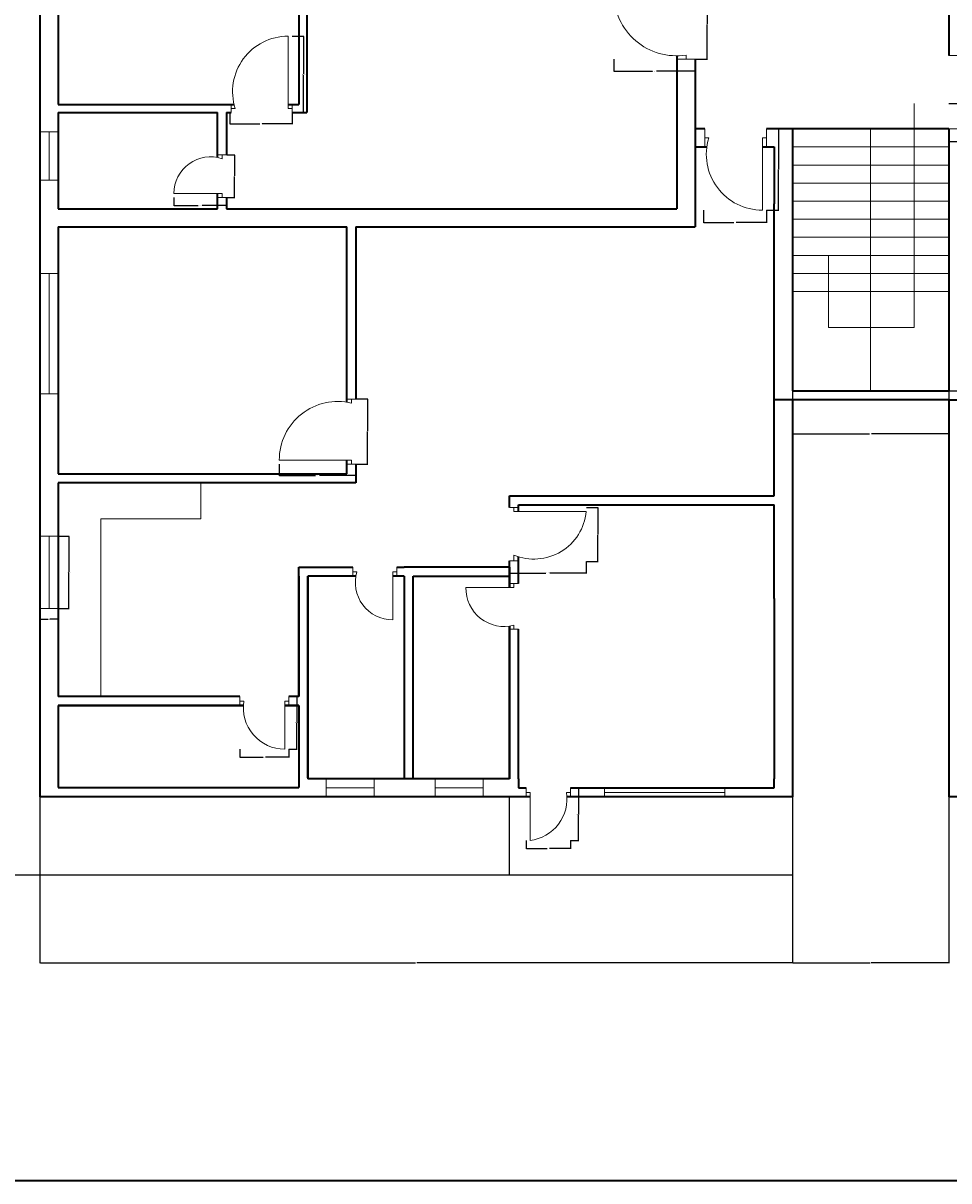
# Model space of a CAD drawing. Units: inches. Extents: x 2120 to 4013, y 1390 to 3019.
# Tile 50 of 59: x 3063 to 3525, y 1390 to 1967. Entities that reach past the tile are written whole.
import ezdxf

# ---------------------------------------------------------------- set-up
doc = ezdxf.new("R2010")
doc.units = ezdxf.units.IN
for name, color, linetype, lineweight in [('A-ANNO-DIMS', 2, 'Continuous', 18), ('A-ANNO-TTLB', 7, 'Continuous', 35), ('A-DOOR', 3, 'Continuous', 18), ('A-FLOR-CASE', 8, 'Continuous', 18), ('A-FLOR-DECK', 7, 'Continuous', 25), ('A-FLOR-STRS', 7, 'Continuous', 18), ('A-FURN', 8, 'Continuous', 13), ('A-GLAZ', 4, 'Continuous', 18), ('A-WALL', 7, 'Continuous', 35)]:
    doc.layers.add(name, color=color, linetype=linetype, lineweight=lineweight)
doc.styles.get("Standard").update_dxf_attribs({"font": 'arial.ttf'})
doc.dimstyles.get("Standard").update_dxf_attribs({"dimtxt": 0.18, "dimasz": 0.18, "dimexe": 0.18, "dimexo": 0.0625, "dimgap": 0.09, "dimtad": 0, "dimtih": 1, "dimtoh": 1, "dimdec": 4, "dimzin": 0, "dimdsep": 46, "dimtxsty": 'Standard', "dimcen": 0.09, "dimadec": 0, "dimazin": 0, "dimtfac": 1, "dimtdec": 4, "dimtofl": 0, "dimtmove": 0, "dimatfit": 3, "dimfxl": 1, "dimtolj": 1, "dimtzin": 0, "dimarcsym": 0})

# ---------------------------------------------------------------- blocks, each defined once
blk = doc.blocks.new('DOOR-SWING-24IN-108p49DEG')
for p, q in [((21.75, 21.28), (26.25, 21.28)), ((26.25, 21.28), (24, 21.28)), ((24, 21.28), (24, 19.28)), ((24, 2), (0, 2)), ((24, 0), (24, 2)), ((26.25, 0), (21.75, 0)), ((21.75, 0), (24, 0))]:
    blk.add_line(p, q)
blk.add_arc((18.22, 2), 18.22, 71.50887, 180)
blk = doc.blocks.new('DOOR-SWING-24IN-91p57DEG')
for p, q in [((0, 26.25), (0, 21.75)), ((0, 21.75), (0, 24)), ((0, 24), (2, 24)), ((2, 24), (2, 0)), ((22.12, 24), (20.12, 24)), ((22.12, 21.75), (22.12, 26.25)), ((22.12, 26.25), (22.12, 24))]:
    blk.add_line(p, q)
blk.add_arc((-0.62, 20.81), 20.98, 277.16426, 8.73852)
blk = doc.blocks.new('DOOR-SWING-24IN-105p55DEG')
for p, q in [((24, 20.82), (0, 20.82)), ((21.75, 22.82), (26.25, 22.82)), ((26.25, 22.82), (24, 22.82)), ((24, 22.82), (24, 20.82)), ((21.75, 0), (26.25, 0)), ((24, 0), (24, 2)), ((26.25, 0), (24, 0))]:
    blk.add_line(p, q)
blk.add_arc((19.15, 20.53), 19.15, 179.12074, 284.67391)
blk = doc.blocks.new('DOOR-SWING-24IN-106p83DEG')
for p, q in [((0, 21.75), (0, 26.25)), ((0, 26.25), (0, 24)), ((0, 24), (2, 24)), ((21.81, 24), (19.81, 24)), ((19.81, 24), (19.81, 0)), ((21.81, 21.75), (21.81, 26.25)), ((21.81, 26.25), (21.81, 24))]:
    blk.add_line(p, q)
blk.add_arc((19.81, 18.61), 18.61, 163.16612, 270)
blk = doc.blocks.new('DOOR-SWING-24IN-99p42DEG')
for p, q in [((0, 26.25), (0, 21.75)), ((0, 21.75), (0, 24)), ((0, 24), (2, 24)), ((24.35, 24), (22.35, 24)), ((22.35, 24), (22.35, 0)), ((24.35, 21.75), (24.35, 26.25)), ((24.35, 26.25), (24.35, 24))]:
    blk.add_line(p, q)
blk.add_arc((22.35, 20.62), 20.62, 170.58134, 270)
blk = doc.blocks.new('DOOR-SWING-36IN-107p46DEG')
for p, q in [((28.42, 2), (28.42, 38)), ((0, 0), (0, 4)), ((0, 4), (0, 2)), ((0, 2), (2, 2)), ((30.42, 2), (28.42, 2)), ((30.42, 4), (30.42, 0)), ((30.42, 0), (30.42, 2))]:
    blk.add_line(p, q)
blk.add_arc((28.42, 10.31), 27.69, 90, 197.45547)
blk = doc.blocks.new('DOOR-SWING-36IN-98p95DEG')
for p, q in [((31.5, 34.77), (40.5, 34.77)), ((40.5, 34.77), (36, 34.77)), ((36, 34.77), (36, 32.77)), ((36, 32.77), (0, 32.77)), ((31.5, 0), (40.5, 0)), ((36, 0), (36, 2)), ((40.5, 0), (36, 0))]:
    blk.add_line(p, q)
blk.add_arc((31.15, 32.77), 31.15, 180, 278.94961)
blk = doc.blocks.new('DOOR-SWING-36IN-109p07DEG')
for p, q in [((9, 36.56), (0, 36.56)), ((0, 36.56), (4.5, 36.56)), ((4.5, 36.56), (4.5, 34.56)), ((9, 36.56), (9, 36.56)), ((4.5, 34.56), (40.5, 34.56)), ((9, 0), (0, 0)), ((0, 0), (4.5, 0)), ((4.5, 0), (4.5, 2))]:
    blk.add_line(p, q)
blk.add_arc((10.9, 31.1), 29.8, 257.59275, 6.66524)
blk = doc.blocks.new('DOOR-SWING-36IN-103p48DEG')
for p, q in [((33.75, 32.39), (38.25, 32.39)), ((38.25, 32.39), (36, 32.39)), ((36, 32.39), (36, 30.39)), ((36, 2), (0, 2)), ((33.75, 0), (38.25, 0)), ((36, 0), (36, 2)), ((38.25, 0), (36, 0))]:
    blk.add_line(p, q)
blk.add_arc((29.19, 2), 29.19, 76.52068, 180)
blk = doc.blocks.new('DOOR-SWING-36IN-107p00DEG')
for p, q in [((4.5, 26.58), (0, 26.58)), ((0, 26.58), (2.25, 26.58)), ((2.25, 26.58), (2.25, 24.58)), ((2.25, 24.58), (38.25, 24.58)), ((4.5, 0), (0, 0)), ((0, 0), (2.25, 0)), ((2.25, 0), (2.25, 2.87))]:
    blk.add_line(p, q)
blk.add_arc((12.22, 27.04), 26.15, 247.59897, 354.59991)
blk = doc.blocks.new('DOOR-SWING-36IN-106p79DEG')
for p, q in [((0, 40.5), (0, 31.5)), ((30.74, 31.5), (30.74, 40.5)), ((30.74, 40.5), (30.74, 36)), ((0, 31.5), (0, 36)), ((0, 36), (2, 36)), ((30.74, 36), (28.74, 36)), ((28.74, 36), (28.74, 0))]:
    blk.add_line(p, q)
blk.add_arc((28.74, 27.93), 27.93, 163.20753, 270)
blk = doc.blocks.new('WIN-PLAN-24IN-03')
for p, q in [((9, 24), (0, 24)), ((0, 24), (4.5, 24)), ((4.5, 24), (4.5, 0)), ((9, 0), (0, 0)), ((4.5, 0), (9, 0))]:
    blk.add_line(p, q)
blk = doc.blocks.new('WIN-PLAN-60IN-02')
for p, q in [((0, 0), (0, 9)), ((0, 9), (0, 4.5)), ((60, 4.5), (60, 9)), ((60, 9), (60, 0)), ((0, 4.5), (60, 4.5))]:
    blk.add_line(p, q)
blk = doc.blocks.new('WIN-PLAN-60IN-05')
for p, q in [((0, 4.5), (0, 0)), ((0, 0), (0, 2.25)), ((0, 2.25), (60, 2.25)), ((60, 2.25), (60, 4.5)), ((60, 4.5), (60, 4.5)), ((60, 4.5), (60, 0))]:
    blk.add_line(p, q)
blk = doc.blocks.new('WIN-PLAN-36IN-03')
for p, q in [((9, 36), (0, 36)), ((0, 36), (4.5, 36)), ((4.5, 36), (4.5, 0)), ((9, 0), (0, 0)), ((4.5, 0), (9, 0))]:
    blk.add_line(p, q)
blk = doc.blocks.new('STAIR-DOGLEG-PLAN')
for p, q in [((60.72, 143.1), (60.72, 31.5)), ((39, 0), (39, 130.5)), ((78, 121.5), (0, 121.5)), ((78, 112.5), (0, 112.5)), ((78, 103.5), (0, 103.5)), ((78, 94.5), (0, 94.5)), ((78, 85.5), (0, 85.5)), ((78, 76.5), (0, 76.5)), ((78, 67.5), (0, 67.5)), ((18.01, 31.5), (18.01, 67.5)), ((78, 58.5), (0, 58.5)), ((78, 49.5), (0, 49.5)), ((60.72, 31.5), (18.01, 31.5)), ((60.72, 31.5), (18.01, 31.5))]:
    blk.add_line(p, q)
blk = doc.blocks.new('*D79')
at = {"layer": 'A-ANNO-DIMS', "color": 0, "lineweight": -2, "transparency": 16777216}
for p, q in [((3524.8, 1926.95), (3546.38, 1926.95)), ((3546.2, 1926.77), (3546.2, 1855.58)), ((3546.2, 1784.02), (3546.2, 1855.21)), ((3524.8, 1783.84), (3546.38, 1783.84))]:
    blk.add_line(p, q, dxfattribs=at)
at = {"layer": 'A-ANNO-DIMS', "color": 0, "transparency": 16777216}
for points in [[(3546.17, 1926.77), (3546.23, 1926.77), (3546.2, 1926.95)], [(3546.17, 1784.02), (3546.23, 1784.02), (3546.2, 1783.84)]]:
    blk.add_solid(points, dxfattribs=at)
at = {"layer": 'Defpoints', "color": 0, "transparency": 16777216}
for p in [(3524.73, 1926.95), (3546.2, 1926.95), (3524.73, 1783.84)]:
    blk.add_point(p, dxfattribs=at)
at = {"layer": 'A-ANNO-DIMS', "color": 0, "transparency": 16777216, "insert": (3546.2, 1855.39), "char_height": 0.18, "attachment_point": 5}
blk.add_mtext('\\A1;STAIR 143 TYP.', dxfattribs=at)
blk = doc.blocks.new('*D80')
at = {"layer": 'A-ANNO-DIMS', "color": 0, "lineweight": -2, "transparency": 16777216}
for p, q in [((3446.73, 1783.78), (3446.73, 1762.2)), ((3524.73, 1783.78), (3524.73, 1762.2)), ((3446.91, 1762.38), (3485.21, 1762.38)), ((3524.55, 1762.38), (3486.26, 1762.38))]:
    blk.add_line(p, q, dxfattribs=at)
at = {"layer": 'A-ANNO-DIMS', "color": 0, "transparency": 16777216}
for points in [[(3446.91, 1762.41), (3446.91, 1762.35), (3446.73, 1762.38)], [(3524.55, 1762.41), (3524.55, 1762.35), (3524.73, 1762.38)]]:
    blk.add_solid(points, dxfattribs=at)
at = {"layer": 'Defpoints', "color": 0, "transparency": 16777216}
for p in [(3446.73, 1783.84), (3524.73, 1783.84), (3524.73, 1762.38)]:
    blk.add_point(p, dxfattribs=at)
at = {"layer": 'A-ANNO-DIMS', "color": 0, "transparency": 16777216, "insert": (3485.73, 1762.38), "char_height": 0.18, "attachment_point": 5}
blk.add_mtext('\\A1;78 TYP.', dxfattribs=at)
blk = doc.blocks.new('*D119')
at = {"layer": 'A-ANNO-DIMS', "color": 0, "lineweight": -2, "transparency": 16777216}
for p, q in [((3138.48, 1880.13), (3138.48, 1876.07)), ((3138.66, 1876.25), (3150.62, 1876.25)), ((3164.55, 1876.25), (3152.6, 1876.25)), ((3164.73, 1880.13), (3164.73, 1876.07))]:
    blk.add_line(p, q, dxfattribs=at)
at = {"layer": 'A-ANNO-DIMS', "color": 0, "transparency": 16777216}
for points in [[(3138.66, 1876.28), (3138.66, 1876.22), (3138.48, 1876.25)], [(3164.55, 1876.28), (3164.55, 1876.22), (3164.73, 1876.25)]]:
    blk.add_solid(points, dxfattribs=at)
at = {"layer": 'Defpoints', "color": 0, "transparency": 16777216}
for p in [(3138.48, 1880.19), (3164.73, 1880.19), (3164.73, 1876.25)]:
    blk.add_point(p, dxfattribs=at)
at = {"layer": 'A-ANNO-DIMS', "color": 0, "transparency": 16777216, "insert": (3151.61, 1876.25), "char_height": 0.18, "attachment_point": 5}
blk.add_mtext('\\A1;SWING 26 TYP.', dxfattribs=at)
blk = doc.blocks.new('*D120')
at = {"layer": 'A-ANNO-DIMS', "color": 0, "lineweight": -2, "transparency": 16777216}
for p, q in [((3164.8, 1901.47), (3168.85, 1901.47)), ((3168.67, 1901.29), (3168.67, 1891.01)), ((3168.67, 1880.37), (3168.67, 1890.65)), ((3164.8, 1880.19), (3168.85, 1880.19))]:
    blk.add_line(p, q, dxfattribs=at)
at = {"layer": 'A-ANNO-DIMS', "color": 0, "transparency": 16777216}
for points in [[(3168.64, 1901.29), (3168.7, 1901.29), (3168.67, 1901.47)], [(3168.64, 1880.37), (3168.7, 1880.37), (3168.67, 1880.19)]]:
    blk.add_solid(points, dxfattribs=at)
at = {"layer": 'Defpoints', "color": 0, "transparency": 16777216}
for p in [(3164.73, 1901.47), (3168.67, 1901.47), (3164.73, 1880.19)]:
    blk.add_point(p, dxfattribs=at)
at = {"layer": 'A-ANNO-DIMS', "color": 0, "transparency": 16777216, "insert": (3168.67, 1890.83), "char_height": 0.18, "attachment_point": 5}
blk.add_mtext('\\A1;21 TYP.', dxfattribs=at)
blk = doc.blocks.new('*D135')
at = {"layer": 'A-ANNO-DIMS', "color": 0, "lineweight": -2, "transparency": 16777216}
for p, q in [((3336.2, 1586.03), (3340.26, 1586.03)), ((3340.08, 1585.85), (3340.08, 1573.09)), ((3340.08, 1559.96), (3340.08, 1572.72)), ((3336.2, 1559.78), (3340.26, 1559.78))]:
    blk.add_line(p, q, dxfattribs=at)
at = {"layer": 'A-ANNO-DIMS', "color": 0, "transparency": 16777216}
for points in [[(3340.05, 1585.85), (3340.11, 1585.85), (3340.08, 1586.03)], [(3340.05, 1559.96), (3340.11, 1559.96), (3340.08, 1559.78)]]:
    blk.add_solid(points, dxfattribs=at)
at = {"layer": 'Defpoints', "color": 0, "transparency": 16777216}
for p in [(3336.14, 1586.03), (3340.08, 1586.03), (3336.14, 1559.78)]:
    blk.add_point(p, dxfattribs=at)
at = {"layer": 'A-ANNO-DIMS', "color": 0, "transparency": 16777216, "insert": (3340.08, 1572.91), "char_height": 0.18, "attachment_point": 5}
blk.add_mtext('\\A1;SWING 26 TYP.', dxfattribs=at)
blk = doc.blocks.new('*D136')
at = {"layer": 'A-ANNO-DIMS', "color": 0, "lineweight": -2, "transparency": 16777216}
for p, q in [((3314.02, 1559.72), (3314.02, 1555.66)), ((3336.14, 1559.72), (3336.14, 1555.66)), ((3314.2, 1555.84), (3324.55, 1555.84)), ((3335.96, 1555.84), (3325.61, 1555.84))]:
    blk.add_line(p, q, dxfattribs=at)
at = {"layer": 'A-ANNO-DIMS', "color": 0, "transparency": 16777216}
for points in [[(3314.2, 1555.87), (3314.2, 1555.81), (3314.02, 1555.84)], [(3335.96, 1555.87), (3335.96, 1555.81), (3336.14, 1555.84)]]:
    blk.add_solid(points, dxfattribs=at)
at = {"layer": 'Defpoints', "color": 0, "transparency": 16777216}
for p in [(3314.02, 1559.78), (3336.14, 1559.78), (3336.14, 1555.84)]:
    blk.add_point(p, dxfattribs=at)
at = {"layer": 'A-ANNO-DIMS', "color": 0, "transparency": 16777216, "insert": (3325.08, 1555.84), "char_height": 0.18, "attachment_point": 5}
blk.add_mtext('\\A1;22 TYP.', dxfattribs=at)
blk = doc.blocks.new('*D141')
at = {"layer": 'A-ANNO-DIMS', "color": 0, "lineweight": -2, "transparency": 16777216}
for p, q in [((3195.81, 1631.53), (3199.86, 1631.53)), ((3199.68, 1631.35), (3199.68, 1618.59)), ((3199.68, 1605.46), (3199.68, 1618.22)), ((3195.81, 1605.28), (3199.86, 1605.28))]:
    blk.add_line(p, q, dxfattribs=at)
at = {"layer": 'A-ANNO-DIMS', "color": 0, "transparency": 16777216}
for points in [[(3199.65, 1631.35), (3199.71, 1631.35), (3199.68, 1631.53)], [(3199.65, 1605.46), (3199.71, 1605.46), (3199.68, 1605.28)]]:
    blk.add_solid(points, dxfattribs=at)
at = {"layer": 'Defpoints', "color": 0, "transparency": 16777216}
for p in [(3195.74, 1631.53), (3199.68, 1631.53), (3195.74, 1605.28)]:
    blk.add_point(p, dxfattribs=at)
at = {"layer": 'A-ANNO-DIMS', "color": 0, "transparency": 16777216, "insert": (3199.68, 1618.41), "char_height": 0.18, "attachment_point": 5}
blk.add_mtext('\\A1;SWING 26 TYP.', dxfattribs=at)
blk = doc.blocks.new('*D142')
at = {"layer": 'A-ANNO-DIMS', "color": 0, "lineweight": -2, "transparency": 16777216}
for p, q in [((3171.4, 1605.22), (3171.4, 1601.16)), ((3195.74, 1605.22), (3195.74, 1601.16)), ((3171.58, 1601.34), (3183.04, 1601.34)), ((3195.56, 1601.34), (3184.1, 1601.34))]:
    blk.add_line(p, q, dxfattribs=at)
at = {"layer": 'A-ANNO-DIMS', "color": 0, "transparency": 16777216}
for points in [[(3171.58, 1601.37), (3171.58, 1601.31), (3171.4, 1601.34)], [(3195.56, 1601.37), (3195.56, 1601.31), (3195.74, 1601.34)]]:
    blk.add_solid(points, dxfattribs=at)
at = {"layer": 'Defpoints', "color": 0, "transparency": 16777216}
for p in [(3171.4, 1605.28), (3195.74, 1605.28), (3195.74, 1601.34)]:
    blk.add_point(p, dxfattribs=at)
at = {"layer": 'A-ANNO-DIMS', "color": 0, "transparency": 16777216, "insert": (3183.57, 1601.34), "char_height": 0.18, "attachment_point": 5}
blk.add_mtext('\\A1;24 TYP.', dxfattribs=at)
blk = doc.blocks.new('*D147')
at = {"layer": 'A-ANNO-DIMS', "color": 0, "lineweight": -2, "transparency": 16777216}
for p, q in [((3197.46, 1960.53), (3203.28, 1960.53)), ((3203.1, 1960.35), (3203.1, 1941.71)), ((3203.1, 1922.71), (3203.1, 1941.35)), ((3197.46, 1922.53), (3203.28, 1922.53))]:
    blk.add_line(p, q, dxfattribs=at)
at = {"layer": 'A-ANNO-DIMS', "color": 0, "transparency": 16777216}
for points in [[(3203.07, 1960.35), (3203.13, 1960.35), (3203.1, 1960.53)], [(3203.07, 1922.71), (3203.13, 1922.71), (3203.1, 1922.53)]]:
    blk.add_solid(points, dxfattribs=at)
at = {"layer": 'Defpoints', "color": 0, "transparency": 16777216}
for p in [(3197.4, 1960.53), (3203.1, 1960.53), (3197.4, 1922.53)]:
    blk.add_point(p, dxfattribs=at)
at = {"layer": 'A-ANNO-DIMS', "color": 0, "transparency": 16777216, "insert": (3203.1, 1941.53), "char_height": 0.18, "attachment_point": 5}
blk.add_mtext('\\A1;SWING 38 TYP.', dxfattribs=at)
blk = doc.blocks.new('*D148')
at = {"layer": 'A-ANNO-DIMS', "color": 0, "lineweight": -2, "transparency": 16777216}
for p, q in [((3166.34, 1922.47), (3166.34, 1916.65)), ((3197.4, 1922.47), (3197.4, 1916.65)), ((3166.52, 1916.83), (3181.34, 1916.83)), ((3197.22, 1916.83), (3182.4, 1916.83))]:
    blk.add_line(p, q, dxfattribs=at)
at = {"layer": 'A-ANNO-DIMS', "color": 0, "transparency": 16777216}
for points in [[(3166.52, 1916.86), (3166.52, 1916.8), (3166.34, 1916.83)], [(3197.22, 1916.86), (3197.22, 1916.8), (3197.4, 1916.83)]]:
    blk.add_solid(points, dxfattribs=at)
at = {"layer": 'Defpoints', "color": 0, "transparency": 16777216}
for p in [(3166.34, 1922.53), (3197.4, 1922.53), (3197.4, 1916.83)]:
    blk.add_point(p, dxfattribs=at)
at = {"layer": 'A-ANNO-DIMS', "color": 0, "transparency": 16777216, "insert": (3181.87, 1916.83), "char_height": 0.18, "attachment_point": 5}
blk.add_mtext('\\A1;31 TYP.', dxfattribs=at)
blk = doc.blocks.new('*D149')
at = {"layer": 'A-ANNO-DIMS', "color": 0, "lineweight": -2, "transparency": 16777216}
for p, q in [((3357.73, 1949.1), (3357.73, 1942.91)), ((3398.23, 1949.1), (3398.23, 1942.91)), ((3357.91, 1943.09), (3377, 1943.09)), ((3398.05, 1943.09), (3378.97, 1943.09))]:
    blk.add_line(p, q, dxfattribs=at)
at = {"layer": 'A-ANNO-DIMS', "color": 0, "transparency": 16777216}
for points in [[(3357.91, 1943.12), (3357.91, 1943.06), (3357.73, 1943.09)], [(3398.05, 1943.12), (3398.05, 1943.06), (3398.23, 1943.09)]]:
    blk.add_solid(points, dxfattribs=at)
at = {"layer": 'Defpoints', "color": 0, "transparency": 16777216}
for p in [(3357.73, 1949.16), (3398.23, 1949.16), (3398.23, 1943.09)]:
    blk.add_point(p, dxfattribs=at)
at = {"layer": 'A-ANNO-DIMS', "color": 0, "transparency": 16777216, "insert": (3377.98, 1943.09), "char_height": 0.18, "attachment_point": 5}
blk.add_mtext('\\A1;SWING 41 TYP.', dxfattribs=at)
blk = doc.blocks.new('*D150')
at = {"layer": 'A-ANNO-DIMS', "color": 0, "lineweight": -2, "transparency": 16777216}
for p, q in [((3398.3, 1983.94), (3404.49, 1983.94)), ((3404.31, 1983.76), (3404.31, 1966.73)), ((3404.31, 1949.34), (3404.31, 1966.37)), ((3398.3, 1949.16), (3404.49, 1949.16))]:
    blk.add_line(p, q, dxfattribs=at)
at = {"layer": 'A-ANNO-DIMS', "color": 0, "transparency": 16777216}
for points in [[(3404.28, 1983.76), (3404.34, 1983.76), (3404.31, 1983.94)], [(3404.28, 1949.34), (3404.34, 1949.34), (3404.31, 1949.16)]]:
    blk.add_solid(points, dxfattribs=at)
at = {"layer": 'Defpoints', "color": 0, "transparency": 16777216}
for p in [(3398.23, 1983.94), (3404.31, 1983.94), (3398.23, 1949.16)]:
    blk.add_point(p, dxfattribs=at)
at = {"layer": 'A-ANNO-DIMS', "color": 0, "transparency": 16777216, "insert": (3404.31, 1966.55), "char_height": 0.18, "attachment_point": 5}
blk.add_mtext('\\A1;35 TYP.', dxfattribs=at)
blk = doc.blocks.new('*D161')
at = {"layer": 'A-ANNO-DIMS', "color": 0, "lineweight": -2, "transparency": 16777216}
for p, q in [((3524.73, 1914.21), (3524.73, 1907.85)), ((3566.35, 1914.21), (3566.35, 1907.85)), ((3524.91, 1908.03), (3544.56, 1908.03)), ((3566.17, 1908.03), (3546.53, 1908.03))]:
    blk.add_line(p, q, dxfattribs=at)
at = {"layer": 'A-ANNO-DIMS', "color": 0, "transparency": 16777216}
for points in [[(3524.91, 1908.06), (3524.91, 1908), (3524.73, 1908.03)], [(3566.17, 1908.06), (3566.17, 1908), (3566.35, 1908.03)]]:
    blk.add_solid(points, dxfattribs=at)
at = {"layer": 'Defpoints', "color": 0, "transparency": 16777216}
for p in [(3524.73, 1914.27), (3566.35, 1914.27), (3566.35, 1908.03)]:
    blk.add_point(p, dxfattribs=at)
at = {"layer": 'A-ANNO-DIMS', "color": 0, "transparency": 16777216, "insert": (3545.54, 1908.03), "char_height": 0.18, "attachment_point": 5}
blk.add_mtext('\\A1;SWING 42 TYP.', dxfattribs=at)
blk = doc.blocks.new('*D163')
at = {"layer": 'A-ANNO-DIMS', "color": 0, "lineweight": -2, "transparency": 16777216}
for p, q in [((3190.98, 1747.28), (3190.98, 1741.42)), ((3229.23, 1747.28), (3229.23, 1741.42)), ((3191.16, 1741.6), (3209.12, 1741.6)), ((3229.05, 1741.6), (3211.1, 1741.6))]:
    blk.add_line(p, q, dxfattribs=at)
at = {"layer": 'A-ANNO-DIMS', "color": 0, "transparency": 16777216}
for points in [[(3191.16, 1741.63), (3191.16, 1741.57), (3190.98, 1741.6)], [(3229.05, 1741.63), (3229.05, 1741.57), (3229.23, 1741.6)]]:
    blk.add_solid(points, dxfattribs=at)
at = {"layer": 'Defpoints', "color": 0, "transparency": 16777216}
for p in [(3190.98, 1747.34), (3229.23, 1747.34), (3229.23, 1741.6)]:
    blk.add_point(p, dxfattribs=at)
at = {"layer": 'A-ANNO-DIMS', "color": 0, "transparency": 16777216, "insert": (3210.11, 1741.6), "char_height": 0.18, "attachment_point": 5}
blk.add_mtext('\\A1;SWING 38 TYP.', dxfattribs=at)
blk = doc.blocks.new('*D164')
at = {"layer": 'A-ANNO-DIMS', "color": 0, "lineweight": -2, "transparency": 16777216}
for p, q in [((3229.3, 1779.81), (3235.15, 1779.81)), ((3234.97, 1779.63), (3234.97, 1763.76)), ((3234.97, 1747.52), (3234.97, 1763.39)), ((3229.3, 1747.34), (3235.15, 1747.34))]:
    blk.add_line(p, q, dxfattribs=at)
at = {"layer": 'A-ANNO-DIMS', "color": 0, "transparency": 16777216}
for points in [[(3234.94, 1779.63), (3235, 1779.63), (3234.97, 1779.81)], [(3234.94, 1747.52), (3235, 1747.52), (3234.97, 1747.34)]]:
    blk.add_solid(points, dxfattribs=at)
at = {"layer": 'Defpoints', "color": 0, "transparency": 16777216}
for p in [(3229.23, 1779.81), (3234.97, 1779.81), (3229.23, 1747.34)]:
    blk.add_point(p, dxfattribs=at)
at = {"layer": 'A-ANNO-DIMS', "color": 0, "transparency": 16777216, "insert": (3234.97, 1763.58), "char_height": 0.18, "attachment_point": 5}
blk.add_mtext('\\A1;32 TYP.', dxfattribs=at)
blk = doc.blocks.new('*D165')
at = {"layer": 'A-ANNO-DIMS', "color": 0, "lineweight": -2, "transparency": 16777216}
for p, q in [((3305.73, 1698.75), (3305.73, 1692.89)), ((3343.98, 1698.75), (3343.98, 1692.89)), ((3305.91, 1693.07), (3323.87, 1693.07)), ((3343.8, 1693.07), (3325.85, 1693.07))]:
    blk.add_line(p, q, dxfattribs=at)
at = {"layer": 'A-ANNO-DIMS', "color": 0, "transparency": 16777216}
for points in [[(3305.91, 1693.1), (3305.91, 1693.04), (3305.73, 1693.07)], [(3343.8, 1693.1), (3343.8, 1693.04), (3343.98, 1693.07)]]:
    blk.add_solid(points, dxfattribs=at)
at = {"layer": 'Defpoints', "color": 0, "transparency": 16777216}
for p in [(3305.73, 1698.81), (3343.98, 1698.81), (3343.98, 1693.07)]:
    blk.add_point(p, dxfattribs=at)
at = {"layer": 'A-ANNO-DIMS', "color": 0, "transparency": 16777216, "insert": (3324.86, 1693.07), "char_height": 0.18, "attachment_point": 5}
blk.add_mtext('\\A1;SWING 38 TYP.', dxfattribs=at)
blk = doc.blocks.new('*D166')
at = {"layer": 'A-ANNO-DIMS', "color": 0, "lineweight": -2, "transparency": 16777216}
for p, q in [((3344.05, 1725.69), (3349.9, 1725.69)), ((3349.72, 1725.51), (3349.72, 1712.43)), ((3349.72, 1698.99), (3349.72, 1712.07)), ((3344.05, 1698.81), (3349.9, 1698.81))]:
    blk.add_line(p, q, dxfattribs=at)
at = {"layer": 'A-ANNO-DIMS', "color": 0, "transparency": 16777216}
for points in [[(3349.69, 1725.51), (3349.75, 1725.51), (3349.72, 1725.69)], [(3349.69, 1698.99), (3349.75, 1698.99), (3349.72, 1698.81)]]:
    blk.add_solid(points, dxfattribs=at)
at = {"layer": 'Defpoints', "color": 0, "transparency": 16777216}
for p in [(3343.98, 1725.69), (3349.72, 1725.69), (3343.98, 1698.81)]:
    blk.add_point(p, dxfattribs=at)
at = {"layer": 'A-ANNO-DIMS', "color": 0, "transparency": 16777216, "insert": (3349.72, 1712.25), "char_height": 0.18, "attachment_point": 5}
blk.add_mtext('\\A1;27 TYP.', dxfattribs=at)
blk = doc.blocks.new('*D167')
at = {"layer": 'A-ANNO-DIMS', "color": 0, "lineweight": -2, "transparency": 16777216}
for p, q in [((3433.83, 1914.34), (3440.03, 1914.34)), ((3439.85, 1914.16), (3439.85, 1894.27)), ((3439.85, 1874.02), (3439.85, 1893.91)), ((3433.83, 1873.84), (3440.03, 1873.84))]:
    blk.add_line(p, q, dxfattribs=at)
at = {"layer": 'A-ANNO-DIMS', "color": 0, "transparency": 16777216}
for points in [[(3439.82, 1914.16), (3439.88, 1914.16), (3439.85, 1914.34)], [(3439.82, 1874.02), (3439.88, 1874.02), (3439.85, 1873.84)]]:
    blk.add_solid(points, dxfattribs=at)
at = {"layer": 'Defpoints', "color": 0, "transparency": 16777216}
for p in [(3433.77, 1914.34), (3439.85, 1914.34), (3433.77, 1873.84)]:
    blk.add_point(p, dxfattribs=at)
at = {"layer": 'A-ANNO-DIMS', "color": 0, "transparency": 16777216, "insert": (3439.85, 1894.09), "char_height": 0.18, "attachment_point": 5}
blk.add_mtext('\\A1;SWING 41 TYP.', dxfattribs=at)
blk = doc.blocks.new('*D168')
at = {"layer": 'A-ANNO-DIMS', "color": 0, "lineweight": -2, "transparency": 16777216}
for p, q in [((3402.48, 1873.78), (3402.48, 1867.59)), ((3433.77, 1873.78), (3433.77, 1867.59)), ((3402.66, 1867.77), (3417.6, 1867.77)), ((3433.59, 1867.77), (3418.65, 1867.77))]:
    blk.add_line(p, q, dxfattribs=at)
at = {"layer": 'A-ANNO-DIMS', "color": 0, "transparency": 16777216}
for points in [[(3402.66, 1867.8), (3402.66, 1867.74), (3402.48, 1867.77)], [(3433.59, 1867.8), (3433.59, 1867.74), (3433.77, 1867.77)]]:
    blk.add_solid(points, dxfattribs=at)
at = {"layer": 'Defpoints', "color": 0, "transparency": 16777216}
for p in [(3402.48, 1873.84), (3433.77, 1873.84), (3433.77, 1867.77)]:
    blk.add_point(p, dxfattribs=at)
at = {"layer": 'A-ANNO-DIMS', "color": 0, "transparency": 16777216, "insert": (3418.13, 1867.77), "char_height": 0.18, "attachment_point": 5}
blk.add_mtext('\\A1;31 TYP.', dxfattribs=at)
blk = doc.blocks.new('*D193')
at = {"layer": 'A-ANNO-DIMS', "color": 0, "lineweight": -2, "transparency": 16777216}
for p, q in [((3080.8, 1711.46), (3086.31, 1711.46)), ((3086.13, 1711.28), (3086.13, 1693.65)), ((3086.13, 1675.64), (3086.13, 1693.28)), ((3080.8, 1675.46), (3086.31, 1675.46))]:
    blk.add_line(p, q, dxfattribs=at)
at = {"layer": 'A-ANNO-DIMS', "color": 0, "transparency": 16777216}
for points in [[(3086.1, 1711.28), (3086.16, 1711.28), (3086.13, 1711.46)], [(3086.1, 1675.64), (3086.16, 1675.64), (3086.13, 1675.46)]]:
    blk.add_solid(points, dxfattribs=at)
at = {"layer": 'Defpoints', "color": 0, "transparency": 16777216}
for p in [(3080.73, 1711.46), (3086.13, 1711.46), (3080.73, 1675.46)]:
    blk.add_point(p, dxfattribs=at)
at = {"layer": 'A-ANNO-DIMS', "color": 0, "transparency": 16777216, "insert": (3086.13, 1693.46), "char_height": 0.18, "attachment_point": 5}
blk.add_mtext('\\A1;WINDOW 36 TYP.', dxfattribs=at)
blk = doc.blocks.new('*D194')
at = {"layer": 'A-ANNO-DIMS', "color": 0, "lineweight": -2, "transparency": 16777216}
for p, q in [((3071.73, 1675.4), (3071.73, 1669.88)), ((3080.73, 1675.4), (3080.73, 1669.88)), ((3071.91, 1670.06), (3075.78, 1670.06)), ((3080.55, 1670.06), (3076.69, 1670.06))]:
    blk.add_line(p, q, dxfattribs=at)
at = {"layer": 'A-ANNO-DIMS', "color": 0, "transparency": 16777216}
for points in [[(3071.91, 1670.09), (3071.91, 1670.03), (3071.73, 1670.06)], [(3080.55, 1670.09), (3080.55, 1670.03), (3080.73, 1670.06)]]:
    blk.add_solid(points, dxfattribs=at)
at = {"layer": 'Defpoints', "color": 0, "transparency": 16777216}
for p in [(3071.73, 1675.46), (3080.73, 1675.46), (3080.73, 1670.06)]:
    blk.add_point(p, dxfattribs=at)
at = {"layer": 'A-ANNO-DIMS', "color": 0, "transparency": 16777216, "insert": (3076.23, 1670.06), "char_height": 0.18, "attachment_point": 5}
blk.add_mtext('\\A1;9 TYP.', dxfattribs=at)
blk = doc.blocks.new('*D217')
at = {"layer": 'A-ANNO-DIMS', "color": 0, "lineweight": -2, "transparency": 16777216}
for p, q in [((3071.67, 2352.53), (2980.31, 2352.53)), ((2980.49, 2352.35), (2980.49, 1947.71)), ((2980.49, 1542.71), (2980.49, 1947.35)), ((3305.67, 1542.53), (2980.31, 1542.53))]:
    blk.add_line(p, q, dxfattribs=at)
at = {"layer": 'A-ANNO-DIMS', "color": 0, "transparency": 16777216}
for points in [[(2980.46, 2352.35), (2980.52, 2352.35), (2980.49, 2352.53)], [(2980.46, 1542.71), (2980.52, 1542.71), (2980.49, 1542.53)]]:
    blk.add_solid(points, dxfattribs=at)
at = {"layer": 'Defpoints', "color": 0, "transparency": 16777216}
for p in [(2980.49, 2352.53), (3071.73, 2352.53), (3305.73, 1542.53)]:
    blk.add_point(p, dxfattribs=at)
at = {"layer": 'A-ANNO-DIMS', "color": 0, "transparency": 16777216, "insert": (2980.49, 1947.53), "char_height": 0.18, "attachment_point": 5}
blk.add_mtext('\\A1;810', dxfattribs=at)
blk = doc.blocks.new('*D220')
at = {"layer": 'A-ANNO-DIMS', "color": 0, "lineweight": -2, "transparency": 16777216}
for p, q in [((3071.73, 1581.47), (3071.73, 1498.6)), ((3446.73, 1542.47), (3446.73, 1498.6)), ((3071.91, 1498.78), (3258.95, 1498.78)), ((3446.55, 1498.78), (3259.52, 1498.78))]:
    blk.add_line(p, q, dxfattribs=at)
at = {"layer": 'A-ANNO-DIMS', "color": 0, "transparency": 16777216}
for points in [[(3071.91, 1498.81), (3071.91, 1498.75), (3071.73, 1498.78)], [(3446.55, 1498.81), (3446.55, 1498.75), (3446.73, 1498.78)]]:
    blk.add_solid(points, dxfattribs=at)
at = {"layer": 'Defpoints', "color": 0, "transparency": 16777216}
for p in [(3071.73, 1581.53), (3446.73, 1542.53), (3446.73, 1498.78)]:
    blk.add_point(p, dxfattribs=at)
at = {"layer": 'A-ANNO-DIMS', "color": 0, "transparency": 16777216, "insert": (3259.23, 1498.78), "char_height": 0.18, "attachment_point": 5}
blk.add_mtext('\\A1;375', dxfattribs=at)
blk = doc.blocks.new('*D221')
at = {"layer": 'A-ANNO-DIMS', "color": 0, "lineweight": -2, "transparency": 16777216}
for p, q in [((3524.73, 1581.47), (3524.73, 1498.6)), ((3446.73, 1542.47), (3446.73, 1498.6)), ((3446.91, 1498.78), (3485.52, 1498.78)), ((3524.55, 1498.78), (3485.95, 1498.78))]:
    blk.add_line(p, q, dxfattribs=at)
at = {"layer": 'A-ANNO-DIMS', "color": 0, "transparency": 16777216}
for points in [[(3446.91, 1498.81), (3446.91, 1498.75), (3446.73, 1498.78)], [(3524.55, 1498.81), (3524.55, 1498.75), (3524.73, 1498.78)]]:
    blk.add_solid(points, dxfattribs=at)
at = {"layer": 'Defpoints', "color": 0, "transparency": 16777216}
for p in [(3524.73, 1581.53), (3446.73, 1542.53), (3524.73, 1498.78)]:
    blk.add_point(p, dxfattribs=at)
at = {"layer": 'A-ANNO-DIMS', "color": 0, "transparency": 16777216, "insert": (3485.73, 1498.78), "char_height": 0.18, "attachment_point": 5}
blk.add_mtext('\\A1;78', dxfattribs=at)

msp = doc.modelspace()

# ---------------------------------------------------------------- linework, layer by layer
at = {"layer": 'A-ANNO-TTLB'}
msp.add_lwpolyline([(2120.4581, 3019.1237), (4012.9334, 3019.1237), (4012.9334, 1390.2222), (2120.4581, 1390.2222)], close=True, dxfattribs=at)
at = {"layer": 'A-FLOR-CASE'}
for p, q in [((3151.8644, 1720.0291), (3151.8644, 1738.031)), ((3102.1064, 1631.531), (3102.1064, 1720.0291)), ((3102.1064, 1720.0291), (3151.8644, 1720.0291))]:
    msp.add_line(p, q, dxfattribs=at)
at = {"layer": 'A-FLOR-DECK'}
for p, q in [((3305.7347, 1542.531), (3305.7347, 1581.531)), ((3446.7347, 1581.531), (3446.7347, 1542.531)), ((3446.7347, 1542.531), (3305.7347, 1542.531))]:
    msp.add_line(p, q, dxfattribs=at)
at = {"layer": 'A-FURN'}
for p, q in [((3080.7347, 1792.2228), (3080.7347, 1840.0131)), ((3437.7347, 1675.519), (3437.7347, 1627.7287))]:
    msp.add_line(p, q, dxfattribs=at)
at = {"layer": 'A-WALL'}
for p, q in [((3071.7347, 2352.531), (3071.7347, 1581.531)), ((3080.7347, 2070.531), (3080.7347, 1926.531)), ((3200.7347, 2070.531), (3200.7347, 1926.531)), ((3204.7347, 1992.531), (3204.7347, 1922.531)), ((3524.7347, 1977.7015), (3524.7347, 1962.531)), ((3524.7347, 1962.531), (3524.7347, 1962.531)), ((3524.7347, 1962.531), (3524.7347, 1950.9035)), ((3389.2347, 1950.7852), (3389.2347, 1874.531)), ((3398.2347, 1949.1625), (3398.2347, 1865.531)), ((3080.7347, 1926.531), (3168.4355, 1926.531)), ((3080.7347, 1922.531), (3160.2347, 1922.531)), ((3080.7347, 1922.531), (3080.7347, 1874.531)), ((3160.2347, 1900.0685), (3160.2347, 1922.531)), ((3164.7347, 1922.531), (3166.9831, 1922.531)), ((3164.7347, 1922.531), (3164.7347, 1901.4728)), ((3195.4009, 1926.531), (3200.7347, 1926.531)), ((3197.4009, 1922.531), (3204.7347, 1922.531)), ((3403.032, 1914.3419), (3398.2347, 1914.3419)), ((3398.2347, 1914.3419), (3398.2347, 1905.3419)), ((3437.7347, 1914.3419), (3433.7716, 1914.3419)), ((3524.7347, 1914.3419), (3437.7347, 1914.3419)), ((3446.7347, 1914.3419), (3446.7347, 1783.8419)), ((3524.7347, 1914.3419), (3524.7347, 1783.8419)), ((3398.2347, 1905.3419), (3404.07, 1905.3419)), ((3431.7716, 1905.3419), (3437.7347, 1905.3419)), ((3437.7347, 1905.3419), (3437.7347, 1876.9918)), ((3160.2347, 1874.531), (3160.2347, 1882.1925)), ((3164.7347, 1880.1925), (3164.7347, 1874.531)), ((3437.7347, 1731.531), (3437.7347, 1876.9918)), ((3080.7347, 1874.531), (3160.2347, 1874.531)), ((3080.7347, 1874.531), (3160.2347, 1874.531)), ((3164.7347, 1874.531), (3389.2347, 1874.531)), ((3164.7347, 1874.531), (3389.2347, 1874.531)), ((3080.7347, 1865.531), (3224.7347, 1865.531)), ((3080.7347, 1865.531), (3080.7347, 1742.531)), ((3080.7347, 1865.531), (3080.7347, 1742.531)), ((3224.7347, 1778.1753), (3224.7347, 1865.531)), ((3229.2347, 1865.531), (3398.2347, 1865.531)), ((3229.2347, 1865.531), (3229.2347, 1779.7286)), ((3446.7347, 1783.8419), (3524.7347, 1783.8419)), ((3446.7347, 1779.3419), (3437.7347, 1779.3419)), ((3446.7347, 1779.3419), (3446.7347, 1680.4206)), ((3524.7347, 1779.3419), (3446.7347, 1779.3419)), ((3524.7347, 1779.3419), (3524.7347, 1581.531)), ((3524.7347, 1779.3419), (3533.7347, 1779.3419)), ((3224.7347, 1742.531), (3224.7347, 1749.338)), ((3080.7347, 1742.531), (3224.7347, 1742.531)), ((3229.2347, 1747.338), (3229.2347, 1742.531)), ((3229.2347, 1742.531), (3229.2347, 1738.031)), ((3080.7347, 1738.031), (3080.7347, 1631.531)), ((3229.2347, 1738.031), (3080.7347, 1738.031)), ((3305.7347, 1725.6876), (3305.7347, 1731.531)), ((3305.7347, 1731.531), (3398.2347, 1731.531)), ((3398.2347, 1731.531), (3437.7347, 1731.531)), ((3446.7347, 1731.531), (3446.7347, 1590.531)), ((3310.2347, 1723.6876), (3310.2347, 1727.031)), ((3310.2347, 1727.031), (3437.7347, 1727.031)), ((3437.7347, 1680.4206), (3437.7347, 1727.031)), ((3200.7347, 1691.4513), (3200.7347, 1695.9513)), ((3200.7347, 1695.9513), (3205.2347, 1695.9513)), ((3200.7347, 1631.531), (3200.7347, 1695.9513)), ((3205.2347, 1695.9513), (3227.7221, 1695.9513)), ((3249.5351, 1695.9513), (3253.2347, 1695.9513)), ((3257.7347, 1695.9513), (3253.2347, 1695.9513)), ((3305.7347, 1695.9513), (3257.7347, 1695.9513)), ((3305.7347, 1685.84), (3305.7347, 1699.1039)), ((3305.7347, 1695.9513), (3305.7347, 1685.84)), ((3310.2347, 1687.84), (3310.2347, 1701.1623)), ((3200.7347, 1691.4513), (3200.7347, 1631.531)), ((3205.2347, 1590.9513), (3205.2347, 1691.4513)), ((3229.1913, 1691.4513), (3205.2347, 1691.4513)), ((3205.2347, 1691.4513), (3205.2347, 1590.531)), ((3253.2347, 1691.4513), (3247.5351, 1691.4513)), ((3253.2347, 1691.4513), (3253.2347, 1590.9513)), ((3257.7347, 1590.9513), (3257.7347, 1691.4513)), ((3257.7347, 1691.4513), (3305.7347, 1691.4513)), ((3437.7347, 1680.4206), (3437.7347, 1590.531)), ((3305.7347, 1666.5726), (3305.7347, 1590.531)), ((3305.7347, 1590.531), (3305.7347, 1666.5726)), ((3310.2347, 1590.531), (3310.2347, 1665.0198)), ((3171.3972, 1631.531), (3080.7347, 1631.531)), ((3080.7347, 1627.031), (3080.7347, 1586.1712)), ((3173.1499, 1627.031), (3080.7347, 1627.031)), ((3080.7347, 1627.031), (3173.1499, 1627.031)), ((3200.7347, 1627.031), (3193.744, 1627.031)), ((3193.744, 1627.031), (3200.7347, 1627.031)), ((3200.7347, 1631.531), (3195.744, 1631.531)), ((3200.7347, 1627.031), (3200.7347, 1590.9513)), ((3200.7347, 1627.031), (3200.7347, 1586.1712)), ((3305.7347, 1590.531), (3205.2347, 1590.531)), ((3305.7347, 1590.531), (3288.7347, 1590.531)), ((3310.2347, 1590.531), (3310.2347, 1586.031)), ((3437.7347, 1586.031), (3437.7347, 1590.531)), ((3446.7347, 1590.531), (3446.7347, 1581.531)), ((3316.0211, 1581.531), (3071.7347, 1581.531)), ((3080.7347, 1586.1712), (3200.7347, 1586.1712)), ((3310.2347, 1586.031), (3314.0211, 1586.031)), ((3446.7347, 1581.531), (3334.3609, 1581.531)), ((3336.1383, 1586.031), (3437.7347, 1586.031)), ((3679.4139, 1581.531), (3524.7347, 1581.531))]:
    msp.add_line(p, q, dxfattribs=at)

# ---------------------------------------------------------------- block references
at = {"layer": 'A-DOOR'}
for name, p in [('DOOR-SWING-36IN-98p95DEG', (3357.7347, 1949.1625)), ('DOOR-SWING-36IN-107p46DEG', (3166.9831, 1922.531)), ('DOOR-SWING-36IN-109p07DEG', (3524.7347, 1914.3419)), ('DOOR-SWING-36IN-106p79DEG', (3403.032, 1873.8419)), ('DOOR-SWING-24IN-108p49DEG', (3138.4847, 1880.1925)), ('DOOR-SWING-36IN-103p48DEG', (3190.9847, 1747.338)), ('DOOR-SWING-36IN-107p00DEG', (3305.7347, 1699.1039)), ('DOOR-SWING-24IN-106p83DEG', (3227.7221, 1669.7013)), ('DOOR-SWING-24IN-105p55DEG', (3283.9824, 1665.0198)), ('DOOR-SWING-24IN-99p42DEG', (3171.3972, 1605.281)), ('DOOR-SWING-24IN-91p57DEG', (3314.0211, 1559.781))]:
    msp.add_blockref(name, p, dxfattribs=at)
at = {"layer": 'A-FLOR-STRS'}
msp.add_blockref('STAIR-DOGLEG-PLAN', (3446.7347, 1783.8419), dxfattribs=at)
at = {"layer": 'A-GLAZ'}
for name, p in [('WIN-PLAN-24IN-03', (3071.7347, 1888.8434)), ('WIN-PLAN-36IN-03', (3071.7347, 1675.4639)), ('WIN-PLAN-60IN-05', (3353.1376, 1581.531))]:
    msp.add_blockref(name, p, dxfattribs=at)
for name, p, rotation in [('WIN-PLAN-60IN-02', (3080.7347, 1782.2909), 89.99999999999935), ('WIN-PLAN-24IN-03', (3238.3047, 1581.531), 90.00000000000144), ('WIN-PLAN-24IN-03', (3292.6719, 1581.531), 89.9999999999993)]:
    msp.add_blockref(name, p, dxfattribs=dict(at, rotation=rotation))

# ---------------------------------------------------------------- dimensions: what is measured, and where the dimension line sits
at = {"layer": 'A-ANNO-DIMS'}
dim = msp.add_linear_dim(base=(2980.4877, 2352.531), p1=(3305.7347, 1542.531), p2=(3071.7347, 2352.531), angle=90, dimstyle='Standard', override={"dimdec": 0, "dimlfac": 1, "dimrnd": 0, "dimzin": 0, "dimdsep": 46, "dimlunit": 2}, dxfattribs=at)
dim.commit()
dim.dimension.update_dxf_attribs({"geometry": '*D217', "text_midpoint": (2980.4877, 1947.531)})
for base, p1, p2, text, picture, middle in [((3404.3097, 1983.9368), (3398.2347, 1949.1625), (3398.2347, 1983.9368), '<> TYP.', '*D150', (3404.3097, 1966.5497)), ((3203.1009, 1960.531), (3197.4009, 1922.531), (3197.4009, 1960.531), 'SWING <> TYP.', '*D147', (3203.1009, 1941.531)), ((3546.2003, 1926.9462), (3524.7347, 1783.8419), (3524.7347, 1926.9462), 'STAIR <> TYP.', '*D79', (3546.2003, 1855.394)), ((3439.8466493584, 1914.3418985366), (3433.7716493584, 1873.8418985366), (3433.7716493584, 1914.3418985366), 'SWING <> TYP.', '*D167', (3439.8466493584, 1894.0918985366)), ((3168.6722, 1901.4728), (3164.7347, 1880.1925), (3164.7347, 1901.4728), '<> TYP.', '*D120', (3168.6722, 1890.8327)), ((3234.9722, 1779.8125), (3229.2347, 1747.338), (3229.2347, 1779.8125), '<> TYP.', '*D164', (3234.9722, 1763.5752)), ((3349.7222, 1725.6876), (3343.9847, 1698.8121), (3343.9847, 1725.6876), '<> TYP.', '*D166', (3349.7222, 1712.2499)), ((3086.1347, 1711.4639), (3080.7347, 1675.4639), (3080.7347, 1711.4639), 'WINDOW <> TYP.', '*D193', (3086.1347, 1693.4639)), ((3199.6815, 1631.531), (3195.744, 1605.281), (3195.744, 1631.531), 'SWING <> TYP.', '*D141', (3199.6815, 1618.406)), ((3340.0758, 1586.031), (3336.1383, 1559.781), (3336.1383, 1586.031), 'SWING <> TYP.', '*D135', (3340.0758, 1572.906))]:
    dim = msp.add_linear_dim(base=base, p1=p1, p2=p2, angle=90, text=text, dimstyle='Standard', override={"dimdec": 0, "dimlfac": 1, "dimrnd": 0, "dimzin": 0, "dimdsep": 46, "dimlunit": 2}, dxfattribs=at)
    dim.commit()
    dim.dimension.update_dxf_attribs({"geometry": picture, "text_midpoint": middle})
for base, p1, p2, text, picture, middle in [((3398.2346645849, 1943.0875170626), (3357.7346645849, 1949.1625170626), (3398.2346645849, 1949.1625170626), 'SWING <> TYP.', '*D149', (3377.9846645849, 1943.0875170626)), ((3197.4009, 1916.831), (3166.3379, 1922.531), (3197.4009, 1922.531), '<> TYP.', '*D148', (3181.8694, 1916.831)), ((3566.3532, 1908.0285), (3524.7347, 1914.2713), (3566.3532, 1914.2713), 'SWING <> TYP.', '*D161', (3545.5439, 1908.0285)), ((3164.7347, 1876.255), (3138.4847, 1880.1925), (3164.7347, 1880.1925), 'SWING <> TYP.', '*D119', (3151.6097, 1876.255)), ((3433.7716, 1867.7669), (3402.4789, 1873.8419), (3433.7716, 1873.8419), '<> TYP.', '*D168', (3418.1253, 1867.7669)), ((3524.7347, 1762.3763), (3446.7347, 1783.8419), (3524.7347, 1783.8419), '<> TYP.', '*D80', (3485.7347, 1762.3763)), ((3229.2347, 1741.6005), (3190.9847, 1747.338), (3229.2347, 1747.338), 'SWING <> TYP.', '*D163', (3210.1097, 1741.6005)), ((3343.9847, 1693.0746), (3305.7347, 1698.8121), (3343.9847, 1698.8121), 'SWING <> TYP.', '*D165', (3324.8597, 1693.0746)), ((3080.7347, 1670.0639), (3071.7347, 1675.4639), (3080.7347, 1675.4639), '<> TYP.', '*D194', (3076.2347, 1670.0639)), ((3195.744, 1601.3435), (3171.3972, 1605.281), (3195.744, 1605.281), '<> TYP.', '*D142', (3183.5706, 1601.3435)), ((3336.1383, 1555.8435), (3314.0211, 1559.781), (3336.1383, 1559.781), '<> TYP.', '*D136', (3325.0797, 1555.8435))]:
    dim = msp.add_linear_dim(base=base, p1=p1, p2=p2, text=text, dimstyle='Standard', override={"dimdec": 0, "dimlfac": 1, "dimrnd": 0, "dimzin": 0, "dimdsep": 46, "dimlunit": 2}, dxfattribs=at)
    dim.commit()
    dim.dimension.update_dxf_attribs({"geometry": picture, "text_midpoint": middle})
for base, p1, p2, picture, middle in [((3446.7347, 1498.781), (3071.7347, 1581.531), (3446.7347, 1542.531), '*D220', (3259.2347, 1498.781)), ((3524.7347, 1498.781), (3446.7347, 1542.531), (3524.7347, 1581.531), '*D221', (3485.7347, 1498.781))]:
    dim = msp.add_linear_dim(base=base, p1=p1, p2=p2, dimstyle='Standard', override={"dimdec": 0, "dimlfac": 1, "dimrnd": 0, "dimzin": 0, "dimdsep": 46, "dimlunit": 2}, dxfattribs=at)
    dim.commit()
    dim.dimension.update_dxf_attribs({"geometry": picture, "text_midpoint": middle})

doc.saveas('drawing.dxf')
